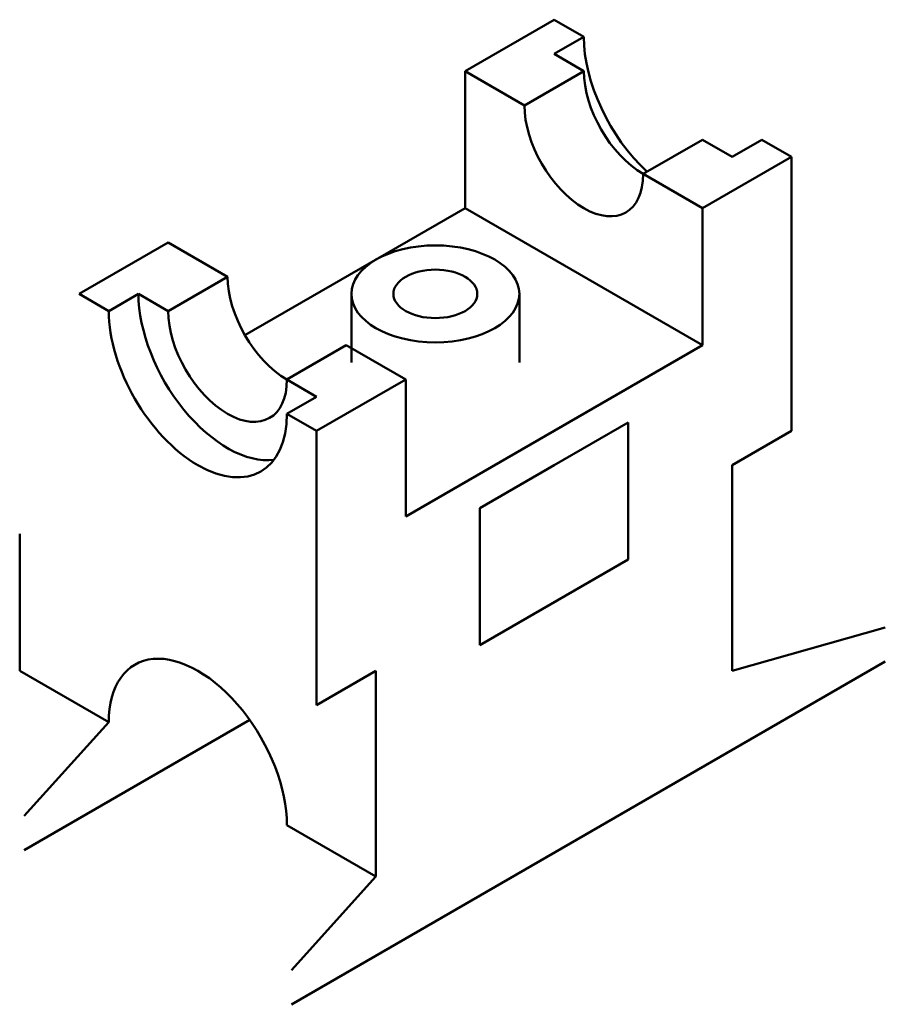
# Model space of a CAD drawing. Units: inches. Extents: x 595 to 18402, y 316 to 10662.
# Tile 1 of 2: x 595 to 721, y 316 to 460. Entities that reach past the tile are written whole.
import ezdxf

# ---------------------------------------------------------------- set-up
doc = ezdxf.new("R2010")
doc.units = ezdxf.units.IN
doc.header["$MEASUREMENT"] = 0
doc.layers.add('M-OUTL', color=7, linetype='Continuous', lineweight=50)

msp = doc.modelspace()

# ---------------------------------------------------------------- linework, layer by layer
at = {"layer": 'M-OUTL'}
for p, q in [((659.53, 452.26), (672.52, 459.76)), ((672.52, 459.76), (676.85, 457.26)), ((676.85, 457.26), (672.52, 454.76)), ((672.52, 454.76), (676.85, 452.26)), ((668.19, 447.26), (659.53, 452.26)), ((659.53, 432.26), (659.53, 452.26)), ((676.85, 452.26), (668.19, 447.26)), ((694.17, 442.26), (685.51, 437.26)), ((698.5, 439.76), (694.17, 442.26)), ((702.83, 442.26), (698.5, 439.76)), ((707.16, 439.76), (702.83, 442.26)), ((694.17, 432.26), (707.16, 439.76)), ((707.16, 399.76), (707.16, 439.76)), ((685.51, 437.26), (694.17, 432.26)), ((659.53, 432.26), (627.42, 413.73)), ((694.17, 412.26), (659.53, 432.26)), ((694.17, 412.26), (694.17, 432.26)), ((603.24, 419.76), (616.23, 427.26)), ((616.23, 427.26), (624.89, 422.26)), ((616.23, 417.26), (624.89, 422.26)), ((607.57, 417.26), (603.24, 419.76)), ((607.57, 417.26), (611.9, 419.76)), ((611.9, 419.76), (616.23, 417.26)), ((642.95, 409.76), (642.95, 419.76)), ((667.45, 409.76), (667.45, 419.76)), ((633.55, 407.26), (642.21, 412.26)), ((642.21, 412.26), (650.87, 407.26)), ((650.87, 387.26), (694.17, 412.26)), ((637.88, 404.76), (633.55, 407.26)), ((637.88, 399.76), (650.87, 407.26)), ((650.87, 407.26), (650.87, 387.26)), ((633.55, 402.26), (637.88, 404.76)), ((637.88, 399.76), (633.55, 402.26)), ((672.52, 394.76), (683.34, 401.01)), ((683.34, 401.01), (683.34, 381.01)), ((637.88, 359.76), (637.88, 399.76)), ((698.5, 394.76), (707.16, 399.76)), ((661.69, 388.51), (672.52, 394.76)), ((698.5, 364.76), (698.5, 394.76)), ((661.69, 368.51), (661.69, 388.51)), ((594.58, 364.76), (594.58, 384.76)), ((683.34, 381.01), (661.69, 368.51)), ((720.82, 371.1), (698.5, 364.76)), ((634.22, 316.1), (720.82, 366.1)), ((607.57, 357.26), (594.58, 364.76)), ((646.54, 364.76), (637.88, 359.76)), ((646.54, 334.76), (646.54, 364.76)), ((595.25, 338.6), (628.13, 357.59)), ((595.25, 343.6), (607.57, 357.26)), ((646.54, 334.76), (633.55, 342.26)), ((634.22, 321.1), (646.54, 334.76))]:
    msp.add_line(p, q, dxfattribs=at)
for centre, major_axis, start_param, end_param in [((689.84, 449.76), (9.19, -15.91), 3.926991, 5.203272), ((685.51, 447.26), (6.12, -10.61), 3.926991, 5.497787), ((676.85, 442.26), (6.12, -10.61), 3.926991, 7.068583), ((633.55, 417.26), (6.12, -10.61), 3.926991, 5.497787), ((624.89, 412.26), (9.19, -15.91), 3.926991, 6.045244), ((620.56, 409.76), (9.19, -15.91), 3.926991, 7.068583), ((624.89, 412.26), (6.12, -10.61), 3.926991, 7.068583), ((620.56, 349.76), (9.19, -15.91), 7.068583, 10.210176)]:
    msp.add_ellipse(centre, major_axis=major_axis, ratio=0.57735, start_param=start_param, end_param=end_param, dxfattribs=at)
for major_axis in [(-12.25, 0), (-6.12, 0)]:
    msp.add_ellipse((655.2, 419.76), major_axis=major_axis, ratio=0.57735, dxfattribs=at)

doc.saveas('drawing.dxf')
